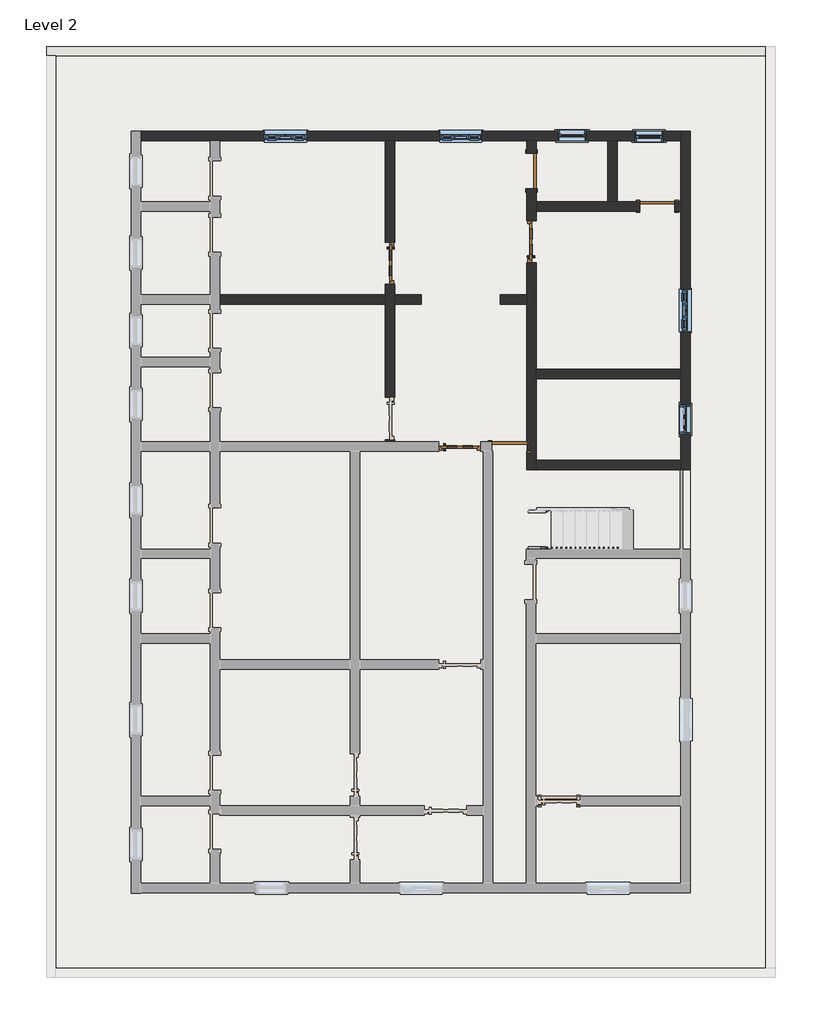
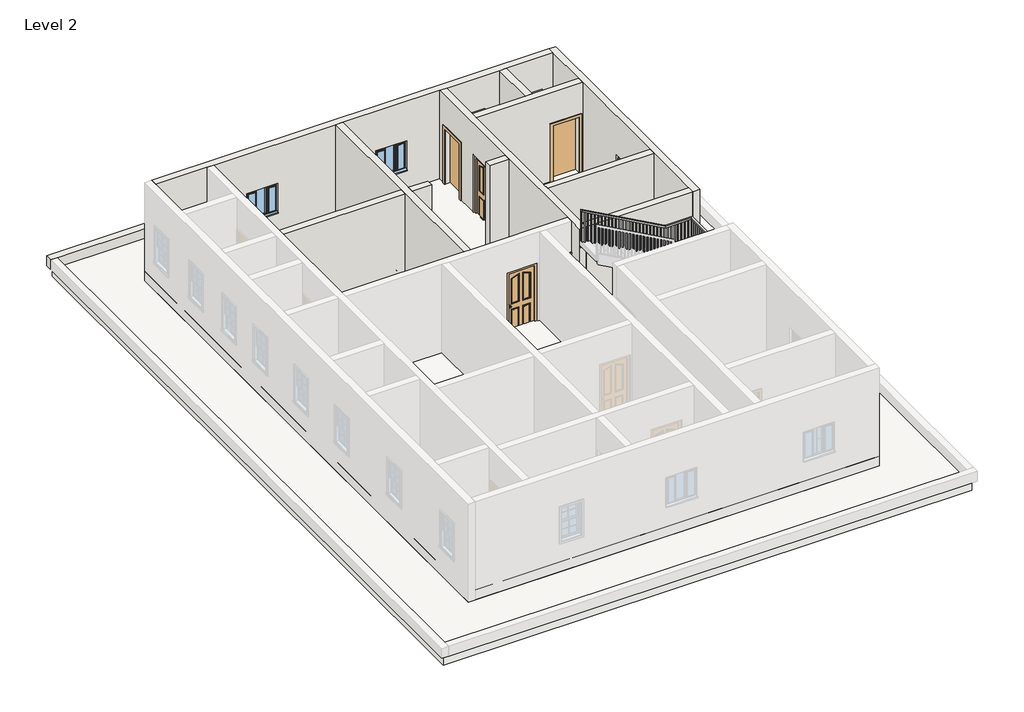
# One storey, part 2 of 3: 11 walls, 6 doors, 6 windows, 2 slabs, 1 railing, 1 roof.
"""IFC4 building model written with IfcOpenShell, lengths in millimetres."""

from ifc_helpers import new_model, si_unit, frame, origin, place, context, project, spatial, polyline, outline, extrude, faceted_brep, transform, mapped, element, save
from components import doors_extsgl_12_910x2110mm_9a09825e, doors_extsgl_12_910x2110mm_ece77ece, door_fadea3f2, window_679d2811, windows_tpl_w_glazing_cross_bars_910x910mm_4aa0f884

model = new_model("IFC4")

# Units and contexts
model_context = context("Model", 3, world=origin())
ifc_project = project(units=[si_unit("LENGTHUNIT", "METRE", prefix="MILLI")], contexts=[model_context])

# Site, building, storey
site = spatial("IfcSite", under=ifc_project)
building = spatial("IfcBuilding", under=site)
storey = spatial("IfcBuildingStorey", under=building, Name="Level 2", Elevation=3048.0)

# Doors
placement = place(None, origin())
doors_extsgl_12_910x2110mm_shape = doors_extsgl_12_910x2110mm_9a09825e(model_context)
element("IfcDoor", 1, ObjectType="Doors_ExtSgl_12 : 910x2110mm", at=placement, inside=storey, context=model_context, shape_type="MappedRepresentation", body=[
    mapped(doors_extsgl_12_910x2110mm_shape, transform((-4887.6876145, 4566.1404944, 3048.0), x_axis=(0.0, -1.0, 0.0), y_axis=(1.0, 0.0, 0.0), z_axis=(0.0, 0.0, 1.0))),
])
element("IfcDoor", 2, ObjectType="Doors_ExtSgl_12 : 910x2110mm", at=placement, inside=storey, context=model_context, shape_type="MappedRepresentation", body=[
    mapped(doors_extsgl_12_910x2110mm_shape, transform((-1839.6876145, 5029.6904944, 3048.0), x_axis=(0.0, 1.0, 0.0), y_axis=(-1.0, 0.0, 0.0), z_axis=(0.0, 0.0, 1.0))),
])
doors_extsgl_12_910x2110mm_2_shape = doors_extsgl_12_910x2110mm_ece77ece(model_context)
element("IfcDoor", 3, ObjectType="Doors_ExtSgl_12 : 910x2110mm", at=placement, inside=storey, context=model_context, shape_type="MappedRepresentation", body=[
    mapped(doors_extsgl_12_910x2110mm_2_shape, transform((-3389.0876145, 603.7404944, 3048.0), x_axis=(1.0, 0.0, 0.0), y_axis=(0.0, 1.0, 0.0), z_axis=(0.0, 0.0, 1.0))),
])
door_shape = door_fadea3f2(model_context)
element("IfcDoor", 4, ObjectType="Single-Flush : 30\" x 80\"", at=placement, inside=storey, context=model_context, shape_type="MappedRepresentation", body=[
    mapped(door_shape, transform((-1839.6876145, 6550.5154944, 3048.0), x_axis=(0.0, -1.0, 0.0), y_axis=(1.0, 0.0, 0.0), z_axis=(0.0, 0.0, 1.0))),
])
element("IfcDoor", 5, ObjectType="Single-Flush : 30\" x 80\"", at=placement, inside=storey, context=model_context, shape_type="MappedRepresentation", body=[
    mapped(door_shape, transform((878.1123855, 5791.6904944, 3048.0), x_axis=(1.0, 0.0, 0.0), y_axis=(0.0, 1.0, 0.0), z_axis=(0.0, 0.0, 1.0))),
])
element("IfcDoor", 6, ObjectType="Single-Flush : 30\" x 80\"", at=placement, inside=storey, context=model_context, shape_type="MappedRepresentation", body=[
    mapped(door_shape, transform((-2309.5876145, 603.7404944, 3048.0), x_axis=(1.0, 0.0, 0.0), y_axis=(0.0, 1.0, 0.0), z_axis=(0.0, 0.0, 1.0))),
])

# Railing
element("IfcRailing", 7, ObjectType="Handrail - Rectangular", at=placement, inside=storey, context=model_context, shape_type="SolidModel", body=[
    faceted_brep([(-1903.1876145, -1555.2595056, 4099.56), (-1903.1876145, -1555.2595056, 4041.4879132), (-1903.1876145, -1606.0595056, 4041.4879132), (-1903.1876145, -1606.0595056, 4099.56), (325.4830625, -1555.2595056, 5334.0), (338.6121628, -1555.2595056, 5283.2), (338.6121628, -1606.0595056, 5283.2), (325.4830625, -1606.0595056, 5334.0), (1322.6123855, -1555.2595056, 5334.0), (1322.6123855, -1555.2595056, 5283.2), (1373.4123855, -1606.0595056, 5283.2), (1373.4123855, -1606.0595056, 5334.0), (1322.6123855, 57.6404944, 5334.0), (1322.6123855, 57.6404944, 5283.2), (1373.4123855, 108.4404944, 5283.2), (1373.4123855, 108.4404944, 5334.0), (573.1131377, 57.6404944, 5334.0), (559.9840375, 57.6404944, 5283.2), (559.9840375, 108.4404944, 5283.2), (573.1131377, 108.4404944, 5334.0), (-1903.1876145, 57.6404944, 6705.6), (-1903.1876145, 108.4404944, 6705.6), (-1903.1876145, 108.4404944, 6647.5279132), (-1903.1876145, 57.6404944, 6647.5279132)], [[[0, 1, 2, 3]], [[1, 0, 4, 5]], [[2, 1, 5, 6]], [[3, 2, 6, 7]], [[0, 3, 7, 4]], [[5, 4, 8, 9]], [[6, 5, 9, 10]], [[7, 6, 10, 11]], [[4, 7, 11, 8]], [[9, 8, 12, 13]], [[10, 9, 13, 14]], [[11, 10, 14, 15]], [[8, 11, 15, 12]], [[13, 12, 16, 17]], [[14, 13, 17, 18]], [[15, 14, 18, 19]], [[12, 15, 19, 16]], [[20, 21, 22, 23]], [[17, 16, 20, 23]], [[18, 17, 23, 22]], [[19, 18, 22, 21]], [[16, 19, 21, 20]]]),
    extrude(outline(polyline([(6585.9768073, -1792.0626145), (6596.5284254, -1811.1126145), (5654.04, -1811.1126145), (5654.04, -1792.0626145), (6585.9768073, -1792.0626145)])), frame((0.0, 73.5154944, 0.0), z_axis=(0.0, 1.0, 0.0), x_axis=(0.0, 0.0, 1.0)), (0.0, 0.0, 1.0), 19.05),
    extrude(outline(polyline([(6529.7015104, -1690.4626145), (6540.2531286, -1709.5126145), (5654.04, -1709.5126145), (5654.04, -1690.4626145), (6529.7015104, -1690.4626145)])), frame((0.0, 73.5154944, 0.0), z_axis=(0.0, 1.0, 0.0), x_axis=(0.0, 0.0, 1.0)), (0.0, 0.0, 1.0), 19.05),
    extrude(outline(polyline([(6473.4262135, -1588.8626145), (6483.9778317, -1607.9126145), (5516.88, -1607.9126145), (5516.88, -1588.8626145), (6473.4262135, -1588.8626145)])), frame((0.0, 73.5154944, 0.0), z_axis=(0.0, 1.0, 0.0), x_axis=(0.0, 0.0, 1.0)), (0.0, 0.0, 1.0), 19.05),
    extrude(outline(polyline([(6417.1509166, -1487.2626145), (6427.7025348, -1506.3126145), (5516.88, -1506.3126145), (5516.88, -1487.2626145), (6417.1509166, -1487.2626145)])), frame((0.0, 73.5154944, 0.0), z_axis=(0.0, 1.0, 0.0), x_axis=(0.0, 0.0, 1.0)), (0.0, 0.0, 1.0), 19.05),
    extrude(outline(polyline([(6360.8756198, -1385.6626145), (6371.4272379, -1404.7126145), (5379.72, -1404.7126145), (5379.72, -1385.6626145), (6360.8756198, -1385.6626145)])), frame((0.0, 73.5154944, 0.0), z_axis=(0.0, 1.0, 0.0), x_axis=(0.0, 0.0, 1.0)), (0.0, 0.0, 1.0), 19.05),
    extrude(outline(polyline([(6304.6003229, -1284.0626145), (6315.151941, -1303.1126145), (5379.72, -1303.1126145), (5379.72, -1284.0626145), (6304.6003229, -1284.0626145)])), frame((0.0, 73.5154944, 0.0), z_axis=(0.0, 1.0, 0.0), x_axis=(0.0, 0.0, 1.0)), (0.0, 0.0, 1.0), 19.05),
    extrude(outline(polyline([(6248.325026, -1182.4626145), (6258.8766442, -1201.5126145), (5379.72, -1201.5126145), (5379.72, -1182.4626145), (6248.325026, -1182.4626145)])), frame((0.0, 73.5154944, 0.0), z_axis=(0.0, 1.0, 0.0), x_axis=(0.0, 0.0, 1.0)), (0.0, 0.0, 1.0), 19.05),
    extrude(outline(polyline([(6192.0497291, -1080.8626145), (6202.6013473, -1099.9126145), (5242.56, -1099.9126145), (5242.56, -1080.8626145), (6192.0497291, -1080.8626145)])), frame((0.0, 73.5154944, 0.0), z_axis=(0.0, 1.0, 0.0), x_axis=(0.0, 0.0, 1.0)), (0.0, 0.0, 1.0), 19.05),
    extrude(outline(polyline([(6135.7744322, -979.2626145), (6146.3260504, -998.3126145), (5242.56, -998.3126145), (5242.56, -979.2626145), (6135.7744322, -979.2626145)])), frame((0.0, 73.5154944, 0.0), z_axis=(0.0, 1.0, 0.0), x_axis=(0.0, 0.0, 1.0)), (0.0, 0.0, 1.0), 19.05),
    extrude(outline(polyline([(6079.4991354, -877.6626145), (6090.0507535, -896.7126145), (5105.4, -896.7126145), (5105.4, -877.6626145), (6079.4991354, -877.6626145)])), frame((0.0, 73.5154944, 0.0), z_axis=(0.0, 1.0, 0.0), x_axis=(0.0, 0.0, 1.0)), (0.0, 0.0, 1.0), 19.05),
    extrude(outline(polyline([(6023.2238385, -776.0626145), (6033.7754566, -795.1126145), (5105.4, -795.1126145), (5105.4, -776.0626145), (6023.2238385, -776.0626145)])), frame((0.0, 73.5154944, 0.0), z_axis=(0.0, 1.0, 0.0), x_axis=(0.0, 0.0, 1.0)), (0.0, 0.0, 1.0), 19.05),
    extrude(outline(polyline([(5966.9485416, -674.4626145), (5977.5001598, -693.5126145), (5105.4, -693.5126145), (5105.4, -674.4626145), (5966.9485416, -674.4626145)])), frame((0.0, 73.5154944, 0.0), z_axis=(0.0, 1.0, 0.0), x_axis=(0.0, 0.0, 1.0)), (0.0, 0.0, 1.0), 19.05),
    extrude(outline(polyline([(5910.6732447, -572.8626145), (5921.2248629, -591.9126145), (4968.24, -591.9126145), (4968.24, -572.8626145), (5910.6732447, -572.8626145)])), frame((0.0, 73.5154944, 0.0), z_axis=(0.0, 1.0, 0.0), x_axis=(0.0, 0.0, 1.0)), (0.0, 0.0, 1.0), 19.05),
    extrude(outline(polyline([(5854.3979478, -471.2626145), (5864.949566, -490.3126145), (4968.24, -490.3126145), (4968.24, -471.2626145), (5854.3979478, -471.2626145)])), frame((0.0, 73.5154944, 0.0), z_axis=(0.0, 1.0, 0.0), x_axis=(0.0, 0.0, 1.0)), (0.0, 0.0, 1.0), 19.05),
    extrude(outline(polyline([(5798.1226509, -369.6626145), (5808.6742691, -388.7126145), (4831.08, -388.7126145), (4831.08, -369.6626145), (5798.1226509, -369.6626145)])), frame((0.0, 73.5154944, 0.0), z_axis=(0.0, 1.0, 0.0), x_axis=(0.0, 0.0, 1.0)), (0.0, 0.0, 1.0), 19.05),
    extrude(outline(polyline([(5741.8473541, -268.0626145), (5752.3989722, -287.1126145), (4831.08, -287.1126145), (4831.08, -268.0626145), (5741.8473541, -268.0626145)])), frame((0.0, 73.5154944, 0.0), z_axis=(0.0, 1.0, 0.0), x_axis=(0.0, 0.0, 1.0)), (0.0, 0.0, 1.0), 19.05),
    extrude(outline(polyline([(5685.5720572, -166.4626145), (5696.1236754, -185.5126145), (4831.08, -185.5126145), (4831.08, -166.4626145), (5685.5720572, -166.4626145)])), frame((0.0, 73.5154944, 0.0), z_axis=(0.0, 1.0, 0.0), x_axis=(0.0, 0.0, 1.0)), (0.0, 0.0, 1.0), 19.05),
    extrude(outline(polyline([(5629.2967603, -64.8626145), (5639.8483785, -83.9126145), (4693.92, -83.9126145), (4693.92, -64.8626145), (5629.2967603, -64.8626145)])), frame((0.0, 73.5154944, 0.0), z_axis=(0.0, 1.0, 0.0), x_axis=(0.0, 0.0, 1.0)), (0.0, 0.0, 1.0), 19.05),
    extrude(outline(polyline([(5573.0214634, 36.7373855), (5583.5730816, 17.6873855), (4693.92, 17.6873855), (4693.92, 36.7373855), (5573.0214634, 36.7373855)])), frame((0.0, 73.5154944, 0.0), z_axis=(0.0, 1.0, 0.0), x_axis=(0.0, 0.0, 1.0)), (0.0, 0.0, 1.0), 19.05),
    extrude(outline(polyline([(5516.7461665, 138.3373855), (5527.2977847, 119.2873855), (4556.76, 119.2873855), (4556.76, 138.3373855), (5516.7461665, 138.3373855)])), frame((0.0, 73.5154944, 0.0), z_axis=(0.0, 1.0, 0.0), x_axis=(0.0, 0.0, 1.0)), (0.0, 0.0, 1.0), 19.05),
    extrude(outline(polyline([(5460.4708697, 239.9373855), (5471.0224878, 220.8873855), (4556.76, 220.8873855), (4556.76, 239.9373855), (5460.4708697, 239.9373855)])), frame((0.0, 73.5154944, 0.0), z_axis=(0.0, 1.0, 0.0), x_axis=(0.0, 0.0, 1.0)), (0.0, 0.0, 1.0), 19.05),
    extrude(outline(polyline([(5404.1955728, 341.5373855), (5414.7471909, 322.4873855), (4419.6, 322.4873855), (4419.6, 341.5373855), (5404.1955728, 341.5373855)])), frame((0.0, 73.5154944, 0.0), z_axis=(0.0, 1.0, 0.0), x_axis=(0.0, 0.0, 1.0)), (0.0, 0.0, 1.0), 19.05),
    extrude(outline(polyline([(5347.9202759, 443.1373855), (5358.4718941, 424.0873855), (4419.6, 424.0873855), (4419.6, 443.1373855), (5347.9202759, 443.1373855)])), frame((0.0, 73.5154944, 0.0), z_axis=(0.0, 1.0, 0.0), x_axis=(0.0, 0.0, 1.0)), (0.0, 0.0, 1.0), 19.05),
    extrude(outline(polyline([(5291.644979, 544.7373855), (5302.1965972, 525.6873855), (4419.6, 525.6873855), (4419.6, 544.7373855), (5291.644979, 544.7373855)])), frame((0.0, 73.5154944, 0.0), z_axis=(0.0, 1.0, 0.0), x_axis=(0.0, 0.0, 1.0)), (0.0, 0.0, 1.0), 19.05),
    extrude(outline(polyline([(646.3373855, 92.5654944), (646.3373855, 73.5154944), (627.2873855, 73.5154944), (627.2873855, 92.5654944), (646.3373855, 92.5654944)])), frame((0.0, 0.0, 4419.6), z_axis=(0.0, 0.0, 1.0), x_axis=(1.0, 0.0, 0.0)), (0.0, 0.0, 1.0), 863.6),
    extrude(outline(polyline([(747.9373855, 92.5654944), (747.9373855, 73.5154944), (728.8873855, 73.5154944), (728.8873855, 92.5654944), (747.9373855, 92.5654944)])), frame((0.0, 0.0, 4419.6), z_axis=(0.0, 0.0, 1.0), x_axis=(1.0, 0.0, 0.0)), (0.0, 0.0, 1.0), 863.6),
    extrude(outline(polyline([(849.5373855, 92.5654944), (849.5373855, 73.5154944), (830.4873855, 73.5154944), (830.4873855, 92.5654944), (849.5373855, 92.5654944)])), frame((0.0, 0.0, 4419.6), z_axis=(0.0, 0.0, 1.0), x_axis=(1.0, 0.0, 0.0)), (0.0, 0.0, 1.0), 863.6),
    extrude(outline(polyline([(951.1373855, 92.5654944), (951.1373855, 73.5154944), (932.0873855, 73.5154944), (932.0873855, 92.5654944), (951.1373855, 92.5654944)])), frame((0.0, 0.0, 4419.6), z_axis=(0.0, 0.0, 1.0), x_axis=(1.0, 0.0, 0.0)), (0.0, 0.0, 1.0), 863.6),
    extrude(outline(polyline([(1052.7373855, 92.5654944), (1052.7373855, 73.5154944), (1033.6873855, 73.5154944), (1033.6873855, 92.5654944), (1052.7373855, 92.5654944)])), frame((0.0, 0.0, 4419.6), z_axis=(0.0, 0.0, 1.0), x_axis=(1.0, 0.0, 0.0)), (0.0, 0.0, 1.0), 863.6),
    extrude(outline(polyline([(1154.3373855, 92.5654944), (1154.3373855, 73.5154944), (1135.2873855, 73.5154944), (1135.2873855, 92.5654944), (1154.3373855, 92.5654944)])), frame((0.0, 0.0, 4419.6), z_axis=(0.0, 0.0, 1.0), x_axis=(1.0, 0.0, 0.0)), (0.0, 0.0, 1.0), 863.6),
    extrude(outline(polyline([(1255.9373855, 92.5654944), (1255.9373855, 73.5154944), (1236.8873855, 73.5154944), (1236.8873855, 92.5654944), (1255.9373855, 92.5654944)])), frame((0.0, 0.0, 4419.6), z_axis=(0.0, 0.0, 1.0), x_axis=(1.0, 0.0, 0.0)), (0.0, 0.0, 1.0), 863.6),
    extrude(outline(polyline([(1357.5373855, 35.4154944), (1338.4873855, 35.4154944), (1338.4873855, 54.4654944), (1357.5373855, 54.4654944), (1357.5373855, 35.4154944)])), frame((0.0, 0.0, 4419.6), z_axis=(0.0, 0.0, 1.0), x_axis=(1.0, 0.0, 0.0)), (0.0, 0.0, 1.0), 863.6),
    extrude(outline(polyline([(1357.5373855, -66.1845056), (1338.4873855, -66.1845056), (1338.4873855, -47.1345056), (1357.5373855, -47.1345056), (1357.5373855, -66.1845056)])), frame((0.0, 0.0, 4419.6), z_axis=(0.0, 0.0, 1.0), x_axis=(1.0, 0.0, 0.0)), (0.0, 0.0, 1.0), 863.6),
    extrude(outline(polyline([(1357.5373855, -167.7845056), (1338.4873855, -167.7845056), (1338.4873855, -148.7345056), (1357.5373855, -148.7345056), (1357.5373855, -167.7845056)])), frame((0.0, 0.0, 4419.6), z_axis=(0.0, 0.0, 1.0), x_axis=(1.0, 0.0, 0.0)), (0.0, 0.0, 1.0), 863.6),
    extrude(outline(polyline([(1357.5373855, -269.3845056), (1338.4873855, -269.3845056), (1338.4873855, -250.3345056), (1357.5373855, -250.3345056), (1357.5373855, -269.3845056)])), frame((0.0, 0.0, 4419.6), z_axis=(0.0, 0.0, 1.0), x_axis=(1.0, 0.0, 0.0)), (0.0, 0.0, 1.0), 863.6),
    extrude(outline(polyline([(1357.5373855, -370.9845056), (1338.4873855, -370.9845056), (1338.4873855, -351.9345056), (1357.5373855, -351.9345056), (1357.5373855, -370.9845056)])), frame((0.0, 0.0, 4419.6), z_axis=(0.0, 0.0, 1.0), x_axis=(1.0, 0.0, 0.0)), (0.0, 0.0, 1.0), 863.6),
    extrude(outline(polyline([(1357.5373855, -472.5845056), (1338.4873855, -472.5845056), (1338.4873855, -453.5345056), (1357.5373855, -453.5345056), (1357.5373855, -472.5845056)])), frame((0.0, 0.0, 4419.6), z_axis=(0.0, 0.0, 1.0), x_axis=(1.0, 0.0, 0.0)), (0.0, 0.0, 1.0), 863.6),
    extrude(outline(polyline([(1357.5373855, -574.1845056), (1338.4873855, -574.1845056), (1338.4873855, -555.1345056), (1357.5373855, -555.1345056), (1357.5373855, -574.1845056)])), frame((0.0, 0.0, 4419.6), z_axis=(0.0, 0.0, 1.0), x_axis=(1.0, 0.0, 0.0)), (0.0, 0.0, 1.0), 863.6),
    extrude(outline(polyline([(1357.5373855, -675.7845056), (1338.4873855, -675.7845056), (1338.4873855, -656.7345056), (1357.5373855, -656.7345056), (1357.5373855, -675.7845056)])), frame((0.0, 0.0, 4419.6), z_axis=(0.0, 0.0, 1.0), x_axis=(1.0, 0.0, 0.0)), (0.0, 0.0, 1.0), 863.6),
    extrude(outline(polyline([(1357.5373855, -777.3845056), (1338.4873855, -777.3845056), (1338.4873855, -758.3345056), (1357.5373855, -758.3345056), (1357.5373855, -777.3845056)])), frame((0.0, 0.0, 4419.6), z_axis=(0.0, 0.0, 1.0), x_axis=(1.0, 0.0, 0.0)), (0.0, 0.0, 1.0), 863.6),
    extrude(outline(polyline([(1357.5373855, -878.9845056), (1338.4873855, -878.9845056), (1338.4873855, -859.9345056), (1357.5373855, -859.9345056), (1357.5373855, -878.9845056)])), frame((0.0, 0.0, 4419.6), z_axis=(0.0, 0.0, 1.0), x_axis=(1.0, 0.0, 0.0)), (0.0, 0.0, 1.0), 863.6),
    extrude(outline(polyline([(1357.5373855, -980.5845056), (1338.4873855, -980.5845056), (1338.4873855, -961.5345056), (1357.5373855, -961.5345056), (1357.5373855, -980.5845056)])), frame((0.0, 0.0, 4419.6), z_axis=(0.0, 0.0, 1.0), x_axis=(1.0, 0.0, 0.0)), (0.0, 0.0, 1.0), 863.6),
    extrude(outline(polyline([(1357.5373855, -1082.1845056), (1338.4873855, -1082.1845056), (1338.4873855, -1063.1345056), (1357.5373855, -1063.1345056), (1357.5373855, -1082.1845056)])), frame((0.0, 0.0, 4419.6), z_axis=(0.0, 0.0, 1.0), x_axis=(1.0, 0.0, 0.0)), (0.0, 0.0, 1.0), 863.6),
    extrude(outline(polyline([(1357.5373855, -1183.7845056), (1338.4873855, -1183.7845056), (1338.4873855, -1164.7345056), (1357.5373855, -1164.7345056), (1357.5373855, -1183.7845056)])), frame((0.0, 0.0, 4419.6), z_axis=(0.0, 0.0, 1.0), x_axis=(1.0, 0.0, 0.0)), (0.0, 0.0, 1.0), 863.6),
    extrude(outline(polyline([(1357.5373855, -1285.3845056), (1338.4873855, -1285.3845056), (1338.4873855, -1266.3345056), (1357.5373855, -1266.3345056), (1357.5373855, -1285.3845056)])), frame((0.0, 0.0, 4419.6), z_axis=(0.0, 0.0, 1.0), x_axis=(1.0, 0.0, 0.0)), (0.0, 0.0, 1.0), 863.6),
    extrude(outline(polyline([(1357.5373855, -1386.9845056), (1338.4873855, -1386.9845056), (1338.4873855, -1367.9345056), (1357.5373855, -1367.9345056), (1357.5373855, -1386.9845056)])), frame((0.0, 0.0, 4419.6), z_axis=(0.0, 0.0, 1.0), x_axis=(1.0, 0.0, 0.0)), (0.0, 0.0, 1.0), 863.6),
    extrude(outline(polyline([(1357.5373855, -1488.5845056), (1338.4873855, -1488.5845056), (1338.4873855, -1469.5345056), (1357.5373855, -1469.5345056), (1357.5373855, -1488.5845056)])), frame((0.0, 0.0, 4419.6), z_axis=(0.0, 0.0, 1.0), x_axis=(1.0, 0.0, 0.0)), (0.0, 0.0, 1.0), 863.6),
    extrude(outline(polyline([(1236.8873855, -1590.1845056), (1236.8873855, -1571.1345056), (1255.9373855, -1571.1345056), (1255.9373855, -1590.1845056), (1236.8873855, -1590.1845056)])), frame((0.0, 0.0, 4419.6), z_axis=(0.0, 0.0, 1.0), x_axis=(1.0, 0.0, 0.0)), (0.0, 0.0, 1.0), 863.6),
    extrude(outline(polyline([(1135.2873855, -1590.1845056), (1135.2873855, -1571.1345056), (1154.3373855, -1571.1345056), (1154.3373855, -1590.1845056), (1135.2873855, -1590.1845056)])), frame((0.0, 0.0, 4419.6), z_axis=(0.0, 0.0, 1.0), x_axis=(1.0, 0.0, 0.0)), (0.0, 0.0, 1.0), 863.6),
    extrude(outline(polyline([(1033.6873855, -1590.1845056), (1033.6873855, -1571.1345056), (1052.7373855, -1571.1345056), (1052.7373855, -1590.1845056), (1033.6873855, -1590.1845056)])), frame((0.0, 0.0, 4419.6), z_axis=(0.0, 0.0, 1.0), x_axis=(1.0, 0.0, 0.0)), (0.0, 0.0, 1.0), 863.6),
    extrude(outline(polyline([(932.0873855, -1590.1845056), (932.0873855, -1571.1345056), (951.1373855, -1571.1345056), (951.1373855, -1590.1845056), (932.0873855, -1590.1845056)])), frame((0.0, 0.0, 4419.6), z_axis=(0.0, 0.0, 1.0), x_axis=(1.0, 0.0, 0.0)), (0.0, 0.0, 1.0), 863.6),
    extrude(outline(polyline([(830.4873855, -1590.1845056), (830.4873855, -1571.1345056), (849.5373855, -1571.1345056), (849.5373855, -1590.1845056), (830.4873855, -1590.1845056)])), frame((0.0, 0.0, 4419.6), z_axis=(0.0, 0.0, 1.0), x_axis=(1.0, 0.0, 0.0)), (0.0, 0.0, 1.0), 863.6),
    extrude(outline(polyline([(728.8873855, -1590.1845056), (728.8873855, -1571.1345056), (747.9373855, -1571.1345056), (747.9373855, -1590.1845056), (728.8873855, -1590.1845056)])), frame((0.0, 0.0, 4419.6), z_axis=(0.0, 0.0, 1.0), x_axis=(1.0, 0.0, 0.0)), (0.0, 0.0, 1.0), 863.6),
    extrude(outline(polyline([(627.2873855, -1590.1845056), (627.2873855, -1571.1345056), (646.3373855, -1571.1345056), (646.3373855, -1590.1845056), (627.2873855, -1590.1845056)])), frame((0.0, 0.0, 4419.6), z_axis=(0.0, 0.0, 1.0), x_axis=(1.0, 0.0, 0.0)), (0.0, 0.0, 1.0), 863.6),
    extrude(outline(polyline([(525.6873855, -1590.1845056), (525.6873855, -1571.1345056), (544.7373855, -1571.1345056), (544.7373855, -1590.1845056), (525.6873855, -1590.1845056)])), frame((0.0, 0.0, 4419.6), z_axis=(0.0, 0.0, 1.0), x_axis=(1.0, 0.0, 0.0)), (0.0, 0.0, 1.0), 863.6),
    extrude(outline(polyline([(424.0873855, -1590.1845056), (424.0873855, -1571.1345056), (443.1373855, -1571.1345056), (443.1373855, -1590.1845056), (424.0873855, -1590.1845056)])), frame((0.0, 0.0, 4419.6), z_axis=(0.0, 0.0, 1.0), x_axis=(1.0, 0.0, 0.0)), (0.0, 0.0, 1.0), 863.6),
    extrude(outline(polyline([(322.4873855, -1590.1845056), (322.4873855, -1571.1345056), (341.5373855, -1571.1345056), (341.5373855, -1590.1845056), (322.4873855, -1590.1845056)])), frame((0.0, 0.0, 4419.6), z_axis=(0.0, 0.0, 1.0), x_axis=(1.0, 0.0, 0.0)), (0.0, 0.0, 1.0), 863.6),
    extrude(outline(polyline([(5228.5449568, 239.9373855), (5217.9933387, 220.8873855), (4282.44, 220.8873855), (4282.44, 239.9373855), (5228.5449568, 239.9373855)])), frame((0.0, -1590.1845056, 0.0), z_axis=(0.0, 1.0, 0.0), x_axis=(0.0, 0.0, 1.0)), (0.0, 0.0, 1.0), 19.05),
    extrude(outline(polyline([(5172.2696599, 138.3373855), (5161.7180418, 119.2873855), (4282.44, 119.2873855), (4282.44, 138.3373855), (5172.2696599, 138.3373855)])), frame((0.0, -1590.1845056, 0.0), z_axis=(0.0, 1.0, 0.0), x_axis=(0.0, 0.0, 1.0)), (0.0, 0.0, 1.0), 19.05),
    extrude(outline(polyline([(5115.9943631, 36.7373855), (5105.4427449, 17.6873855), (4145.28, 17.6873855), (4145.28, 36.7373855), (5115.9943631, 36.7373855)])), frame((0.0, -1590.1845056, 0.0), z_axis=(0.0, 1.0, 0.0), x_axis=(0.0, 0.0, 1.0)), (0.0, 0.0, 1.0), 19.05),
    extrude(outline(polyline([(5059.7190662, -64.8626145), (5049.167448, -83.9126145), (4145.28, -83.9126145), (4145.28, -64.8626145), (5059.7190662, -64.8626145)])), frame((0.0, -1590.1845056, 0.0), z_axis=(0.0, 1.0, 0.0), x_axis=(0.0, 0.0, 1.0)), (0.0, 0.0, 1.0), 19.05),
    extrude(outline(polyline([(5003.4437693, -166.4626145), (4992.8921511, -185.5126145), (4008.12, -185.5126145), (4008.12, -166.4626145), (5003.4437693, -166.4626145)])), frame((0.0, -1590.1845056, 0.0), z_axis=(0.0, 1.0, 0.0), x_axis=(0.0, 0.0, 1.0)), (0.0, 0.0, 1.0), 19.05),
    extrude(outline(polyline([(4947.1684724, -268.0626145), (4936.6168543, -287.1126145), (4008.12, -287.1126145), (4008.12, -268.0626145), (4947.1684724, -268.0626145)])), frame((0.0, -1590.1845056, 0.0), z_axis=(0.0, 1.0, 0.0), x_axis=(0.0, 0.0, 1.0)), (0.0, 0.0, 1.0), 19.05),
    extrude(outline(polyline([(4890.8931755, -369.6626145), (4880.3415574, -388.7126145), (4008.12, -388.7126145), (4008.12, -369.6626145), (4890.8931755, -369.6626145)])), frame((0.0, -1590.1845056, 0.0), z_axis=(0.0, 1.0, 0.0), x_axis=(0.0, 0.0, 1.0)), (0.0, 0.0, 1.0), 19.05),
    extrude(outline(polyline([(4834.6178787, -471.2626145), (4824.0662605, -490.3126145), (3870.96, -490.3126145), (3870.96, -471.2626145), (4834.6178787, -471.2626145)])), frame((0.0, -1590.1845056, 0.0), z_axis=(0.0, 1.0, 0.0), x_axis=(0.0, 0.0, 1.0)), (0.0, 0.0, 1.0), 19.05),
    extrude(outline(polyline([(4778.3425818, -572.8626145), (4767.7909636, -591.9126145), (3870.96, -591.9126145), (3870.96, -572.8626145), (4778.3425818, -572.8626145)])), frame((0.0, -1590.1845056, 0.0), z_axis=(0.0, 1.0, 0.0), x_axis=(0.0, 0.0, 1.0)), (0.0, 0.0, 1.0), 19.05),
    extrude(outline(polyline([(4722.0672849, -674.4626145), (4711.5156667, -693.5126145), (3733.8, -693.5126145), (3733.8, -674.4626145), (4722.0672849, -674.4626145)])), frame((0.0, -1590.1845056, 0.0), z_axis=(0.0, 1.0, 0.0), x_axis=(0.0, 0.0, 1.0)), (0.0, 0.0, 1.0), 19.05),
    extrude(outline(polyline([(4665.791988, -776.0626145), (4655.2403699, -795.1126145), (3733.8, -795.1126145), (3733.8, -776.0626145), (4665.791988, -776.0626145)])), frame((0.0, -1590.1845056, 0.0), z_axis=(0.0, 1.0, 0.0), x_axis=(0.0, 0.0, 1.0)), (0.0, 0.0, 1.0), 19.05),
    extrude(outline(polyline([(4609.5166911, -877.6626145), (4598.965073, -896.7126145), (3733.8, -896.7126145), (3733.8, -877.6626145), (4609.5166911, -877.6626145)])), frame((0.0, -1590.1845056, 0.0), z_axis=(0.0, 1.0, 0.0), x_axis=(0.0, 0.0, 1.0)), (0.0, 0.0, 1.0), 19.05),
    extrude(outline(polyline([(4553.2413943, -979.2626145), (4542.6897761, -998.3126145), (3596.64, -998.3126145), (3596.64, -979.2626145), (4553.2413943, -979.2626145)])), frame((0.0, -1590.1845056, 0.0), z_axis=(0.0, 1.0, 0.0), x_axis=(0.0, 0.0, 1.0)), (0.0, 0.0, 1.0), 19.05),
    extrude(outline(polyline([(4496.9660974, -1080.8626145), (4486.4144792, -1099.9126145), (3596.64, -1099.9126145), (3596.64, -1080.8626145), (4496.9660974, -1080.8626145)])), frame((0.0, -1590.1845056, 0.0), z_axis=(0.0, 1.0, 0.0), x_axis=(0.0, 0.0, 1.0)), (0.0, 0.0, 1.0), 19.05),
    extrude(outline(polyline([(4440.6908005, -1182.4626145), (4430.1391823, -1201.5126145), (3459.48, -1201.5126145), (3459.48, -1182.4626145), (4440.6908005, -1182.4626145)])), frame((0.0, -1590.1845056, 0.0), z_axis=(0.0, 1.0, 0.0), x_axis=(0.0, 0.0, 1.0)), (0.0, 0.0, 1.0), 19.05),
    extrude(outline(polyline([(4384.4155036, -1284.0626145), (4373.8638855, -1303.1126145), (3459.48, -1303.1126145), (3459.48, -1284.0626145), (4384.4155036, -1284.0626145)])), frame((0.0, -1590.1845056, 0.0), z_axis=(0.0, 1.0, 0.0), x_axis=(0.0, 0.0, 1.0)), (0.0, 0.0, 1.0), 19.05),
    extrude(outline(polyline([(4328.1402067, -1385.6626145), (4317.5885886, -1404.7126145), (3459.48, -1404.7126145), (3459.48, -1385.6626145), (4328.1402067, -1385.6626145)])), frame((0.0, -1590.1845056, 0.0), z_axis=(0.0, 1.0, 0.0), x_axis=(0.0, 0.0, 1.0)), (0.0, 0.0, 1.0), 19.05),
    extrude(outline(polyline([(4271.8649099, -1487.2626145), (4261.3132917, -1506.3126145), (3322.32, -1506.3126145), (3322.32, -1487.2626145), (4271.8649099, -1487.2626145)])), frame((0.0, -1590.1845056, 0.0), z_axis=(0.0, 1.0, 0.0), x_axis=(0.0, 0.0, 1.0)), (0.0, 0.0, 1.0), 19.05),
    extrude(outline(polyline([(4215.589613, -1588.8626145), (4205.0379948, -1607.9126145), (3322.32, -1607.9126145), (3322.32, -1588.8626145), (4215.589613, -1588.8626145)])), frame((0.0, -1590.1845056, 0.0), z_axis=(0.0, 1.0, 0.0), x_axis=(0.0, 0.0, 1.0)), (0.0, 0.0, 1.0), 19.05),
    extrude(outline(polyline([(4159.3143161, -1690.4626145), (4148.7626979, -1709.5126145), (3185.16, -1709.5126145), (3185.16, -1690.4626145), (4159.3143161, -1690.4626145)])), frame((0.0, -1590.1845056, 0.0), z_axis=(0.0, 1.0, 0.0), x_axis=(0.0, 0.0, 1.0)), (0.0, 0.0, 1.0), 19.05),
    extrude(outline(polyline([(4103.0390192, -1792.0626145), (4092.487401, -1811.1126145), (3185.16, -1811.1126145), (3185.16, -1792.0626145), (4103.0390192, -1792.0626145)])), frame((0.0, -1590.1845056, 0.0), z_axis=(0.0, 1.0, 0.0), x_axis=(0.0, 0.0, 1.0)), (0.0, 0.0, 1.0), 19.05),
    extrude(outline(polyline([(1357.5373855, 73.5154944), (1338.4873855, 73.5154944), (1338.4873855, 92.5654944), (1357.5373855, 92.5654944), (1357.5373855, 73.5154944)])), frame((0.0, 0.0, 4419.6), z_axis=(0.0, 0.0, 1.0), x_axis=(1.0, 0.0, 0.0)), (0.0, 0.0, 1.0), 863.6),
    extrude(outline(polyline([(1338.4873855, -1590.1845056), (1338.4873855, -1571.1345056), (1357.5373855, -1571.1345056), (1357.5373855, -1590.1845056), (1338.4873855, -1590.1845056)])), frame((0.0, 0.0, 4419.6), z_axis=(0.0, 0.0, 1.0), x_axis=(1.0, 0.0, 0.0)), (0.0, 0.0, 1.0), 863.6),
    extrude(outline(polyline([(6636.9762951, -1884.1376145), (6647.5279132, -1903.1876145), (5654.04, -1903.1876145), (5654.04, -1884.1376145), (6636.9762951, -1884.1376145)])), frame((0.0, 73.5154944, 0.0), z_axis=(0.0, 1.0, 0.0), x_axis=(0.0, 0.0, 1.0)), (0.0, 0.0, 1.0), 19.05),
    extrude(outline(polyline([(4052.0395314, -1884.1376145), (4041.4879132, -1903.1876145), (3185.16, -1903.1876145), (3185.16, -1884.1376145), (4052.0395314, -1884.1376145)])), frame((0.0, -1590.1845056, 0.0), z_axis=(0.0, 1.0, 0.0), x_axis=(0.0, 0.0, 1.0)), (0.0, 0.0, 1.0), 19.05),
])

# Roof
element("IfcRoof", 8, ObjectType="Generic - 12\"", at=placement, inside=storey, context=model_context, shape_type="SweptSolid", body=[
    extrude(outline(polyline([(-10475.6876145, 7410.9404944), (1589.3123855, 7410.9404944), (1589.3123855, -9022.8595056), (-10475.6876145, -9022.8595056), (-10475.6876145, 7410.9404944)])), frame((0.0, 0.0, 3048.0), z_axis=(0.0, 0.0, 1.0), x_axis=(1.0, 0.0, 0.0)), (0.0, 0.0, 1.0), 304.8),
])

# Slabs
element("IfcSlab", 9, ObjectType="Generic - 12\"", at=placement, inside=storey, context=model_context, shape_type="SweptSolid", body=[
    extrude(outline(polyline([(1589.3123855, 7410.9404944), (1589.3123855, -9022.8595056), (-10475.6876145, -9022.8595056), (-10475.6876145, 7410.9404944), (1589.3123855, 7410.9404944)])), frame((0.0, 0.0, 2743.2), z_axis=(0.0, 0.0, 1.0), x_axis=(1.0, 0.0, 0.0)), (0.0, 0.0, 1.0), 304.8),
])
element("IfcSlab", 10, ObjectType="Generic - 12\"", at=placement, inside=storey, context=model_context, shape_type="SweptSolid", body=[
    extrude(outline(polyline([(3316.5123855, 9138.1404944), (3316.5123855, -10750.0595056), (-12202.8876145, -10750.0595056), (-12202.8876145, 9138.1404944), (3316.5123855, 9138.1404944)])), frame((0.0, 0.0, 2743.2), z_axis=(0.0, 0.0, 1.0), x_axis=(1.0, 0.0, 0.0)), (0.0, 0.0, 1.0), 304.8),
])

# Walls
element("IfcWall", 11, ObjectType="4.5\"", at=placement, inside=storey, context=model_context, shape_type="Brep", body=[
    faceted_brep([(-4989.2876145, 758.3404944, 5158.0), (-4989.2876145, 758.3404944, 3048.0), (-4989.2876145, 705.3404944, 3048.0), (-4989.2876145, 705.3404944, 6096.0), (-4989.2876145, 3677.1404944, 6096.0), (-4989.2876145, 3880.3404944, 6096.0), (-4989.2876145, 7207.7404944, 6096.0), (-4989.2876145, 7207.7404944, 3048.0), (-4989.2876145, 5021.1404944, 3048.0), (-4989.2876145, 5021.1404944, 5158.0), (-4989.2876145, 4111.1404944, 5158.0), (-4989.2876145, 4111.1404944, 3048.0), (-4989.2876145, 3880.3404944, 3048.0), (-4989.2876145, 3677.1404944, 3048.0), (-4989.2876145, 1668.3404944, 3048.0), (-4989.2876145, 1668.3404944, 5158.0), (-4786.0876145, 705.3404944, 3048.0), (-4786.0876145, 758.3404944, 3048.0), (-4786.0876145, 758.3404944, 5158.0), (-4786.0876145, 1668.3404944, 5158.0), (-4786.0876145, 1668.3404944, 3048.0), (-4786.0876145, 3677.1404944, 3048.0), (-4786.0876145, 3880.3404944, 3048.0), (-4786.0876145, 4111.1404944, 3048.0), (-4786.0876145, 4111.1404944, 5158.0), (-4786.0876145, 5021.1404944, 5158.0), (-4786.0876145, 5021.1404944, 3048.0), (-4786.0876145, 7207.7404944, 3048.0), (-4786.0876145, 7207.7404944, 6096.0), (-4786.0876145, 3880.3404944, 6096.0), (-4786.0876145, 3677.1404944, 6096.0), (-4786.0876145, 705.3404944, 6096.0)], [[[0, 1, 2, 3, 4, 5, 6, 7, 8, 9, 10, 11, 12, 13, 14, 15]], [[16, 17, 18, 19, 20, 21, 22, 23, 24, 25, 26, 27, 28, 29, 30, 31]], [[8, 7, 27, 26]], [[2, 1, 17, 16]], [[14, 13, 12, 11, 23, 22, 21, 20]], [[6, 5, 4, 3, 31, 30, 29, 28]], [[7, 6, 28, 27]], [[3, 2, 16, 31]], [[26, 25, 9, 8]], [[24, 23, 11, 10]], [[25, 24, 10, 9]], [[20, 19, 15, 14]], [[18, 17, 1, 0]], [[19, 18, 0, 15]]]),
])
element("IfcWall", 12, ObjectType="4.5\"", at=placement, inside=storey, context=model_context, shape_type="SweptSolid", body=[
    extrude(outline(polyline([(-4214.5876145, 3880.3404944), (-4214.5876145, 3677.1404944), (-4786.0876145, 3677.1404944), (-4786.0876145, 3880.3404944), (-4214.5876145, 3880.3404944)])), frame((0.0, 0.0, 3048.0), z_axis=(0.0, 0.0, 1.0), x_axis=(1.0, 0.0, 0.0)), (0.0, 0.0, 1.0), 3048.0),
    extrude(outline(polyline([(-8570.6876145, 3677.1404944), (-8570.6876145, 3880.3404944), (-4989.2876145, 3880.3404944), (-4989.2876145, 3677.1404944), (-8570.6876145, 3677.1404944)])), frame((0.0, 0.0, 3048.0), z_axis=(0.0, 0.0, 1.0), x_axis=(1.0, 0.0, 0.0)), (0.0, 0.0, 1.0), 3048.0),
])
element("IfcWall", 13, ObjectType="4.5\"", at=placement, inside=storey, context=model_context, shape_type="Brep", body=[
    faceted_brep([(-1941.2876145, 6169.5154944, 3048.0), (-1941.2876145, 5484.6904944, 3048.0), (-1941.2876145, 5484.6904944, 5158.0), (-1941.2876145, 4574.6904944, 5158.0), (-1941.2876145, 4574.6904944, 3048.0), (-1941.2876145, 3880.3404944, 3048.0), (-1941.2876145, 3677.1404944, 3048.0), (-1941.2876145, 705.3404944, 3048.0), (-1941.2876145, 705.3404944, 5080.0), (-1941.2876145, 502.1404944, 5080.0), (-1941.2876145, 502.1404944, 3048.0), (-1941.2876145, 108.4404944, 3048.0), (-1941.2876145, 108.4404944, 6096.0), (-1941.2876145, 502.1404944, 6096.0), (-1941.2876145, 705.3404944, 6096.0), (-1941.2876145, 3677.1404944, 6096.0), (-1941.2876145, 3880.3404944, 6096.0), (-1941.2876145, 7207.7404944, 6096.0), (-1941.2876145, 7207.7404944, 3048.0), (-1941.2876145, 6931.5154944, 3048.0), (-1941.2876145, 6931.5154944, 5080.0), (-1941.2876145, 6169.5154944, 5080.0), (-1738.0876145, 5484.6904944, 5158.0), (-1738.0876145, 5484.6904944, 3048.0), (-1738.0876145, 5690.0904944, 3048.0), (-1738.0876145, 5893.2904944, 3048.0), (-1738.0876145, 6169.5154944, 3048.0), (-1738.0876145, 6169.5154944, 5080.0), (-1738.0876145, 6931.5154944, 5080.0), (-1738.0876145, 6931.5154944, 3048.0), (-1738.0876145, 7207.7404944, 3048.0), (-1738.0876145, 7207.7404944, 6096.0), (-1738.0876145, 5893.2904944, 6096.0), (-1738.0876145, 5690.0904944, 6096.0), (-1738.0876145, 2272.4885783, 6096.0), (-1738.0876145, 2069.2885783, 6096.0), (-1738.0876145, 311.6404944, 6096.0), (-1738.0876145, 108.4404944, 6096.0), (-1738.0876145, 108.4404944, 3048.0), (-1738.0876145, 311.6404944, 3048.0), (-1738.0876145, 2069.2885783, 3048.0), (-1738.0876145, 2272.4885783, 3048.0), (-1738.0876145, 4574.6904944, 3048.0), (-1738.0876145, 4574.6904944, 5158.0), (-1928.5876145, 502.1404944, 3048.0), (-1928.5876145, 705.3404944, 3048.0), (-1928.5876145, 502.1404944, 5080.0), (-1928.5876145, 705.3404944, 5080.0)], [[[0, 1, 2, 3, 4, 5, 6, 7, 8, 9, 10, 11, 12, 13, 14, 15, 16, 17, 18, 19, 20, 21]], [[22, 23, 24, 25, 26, 27, 28, 29, 30, 31, 32, 33, 34, 35, 36, 37, 38, 39, 40, 41, 42, 43]], [[18, 30, 29, 19]], [[42, 41, 40, 39, 38, 11, 10, 44, 45, 7, 6, 5, 4]], [[26, 25, 24, 23, 1, 0]], [[17, 16, 15, 14, 13, 12, 37, 36, 35, 34, 33, 32, 31]], [[18, 17, 31, 30]], [[12, 11, 38, 37]], [[27, 26, 0, 21]], [[28, 27, 21, 20]], [[29, 28, 20, 19]], [[46, 44, 10, 9]], [[45, 47, 8, 7]], [[44, 46, 47, 45]], [[47, 46, 9, 8]], [[4, 3, 43, 42]], [[2, 1, 23, 22]], [[3, 2, 22, 43]]]),
])
element("IfcWall", 14, ObjectType="4.5\"", at=placement, inside=storey, context=model_context, shape_type="SweptSolid", body=[
    extrude(outline(polyline([(-2512.7876145, 3880.3404944), (-1941.2876145, 3880.3404944), (-1941.2876145, 3677.1404944), (-2512.7876145, 3677.1404944), (-2512.7876145, 3880.3404944)])), frame((0.0, 0.0, 3048.0), z_axis=(0.0, 0.0, 1.0), x_axis=(1.0, 0.0, 0.0)), (0.0, 0.0, 1.0), 3048.0),
])
element("IfcWall", 15, ObjectType="4.5\"", at=placement, inside=storey, context=model_context, shape_type="SweptSolid", body=[
    extrude(outline(polyline([(1386.1123855, 108.4404944), (-1738.0876145, 108.4404944), (-1738.0876145, 311.6404944), (1386.1123855, 311.6404944), (1386.1123855, 108.4404944)])), frame((0.0, 0.0, 3048.0), z_axis=(0.0, 0.0, 1.0), x_axis=(1.0, 0.0, 0.0)), (0.0, 0.0, 1.0), 3048.0),
])
element("IfcWall", 16, ObjectType="4.5\"", at=placement, inside=storey, context=model_context, shape_type="SweptSolid", body=[
    extrude(outline(polyline([(1386.1123855, 2069.2885783), (-1738.0876145, 2069.2885783), (-1738.0876145, 2272.4885783), (1386.1123855, 2272.4885783), (1386.1123855, 2069.2885783)])), frame((0.0, 0.0, 3048.0), z_axis=(0.0, 0.0, 1.0), x_axis=(1.0, 0.0, 0.0)), (0.0, 0.0, 1.0), 3048.0),
])
element("IfcWall", 17, ObjectType="4.5\"", at=placement, inside=storey, context=model_context, shape_type="Brep", body=[
    faceted_brep([(1259.1123855, 5690.0904944, 5080.0), (1259.1123855, 5690.0904944, 3048.0), (1386.1123855, 5690.0904944, 3048.0), (1386.1123855, 5690.0904944, 6096.0), (-1738.0876145, 5690.0904944, 6096.0), (-1738.0876145, 5690.0904944, 3048.0), (497.1123855, 5690.0904944, 3048.0), (497.1123855, 5690.0904944, 5080.0), (1386.1123855, 5893.2904944, 3048.0), (1259.1123855, 5893.2904944, 3048.0), (1259.1123855, 5893.2904944, 5080.0), (497.1123855, 5893.2904944, 5080.0), (497.1123855, 5893.2904944, 3048.0), (14.5123855, 5893.2904944, 3048.0), (-188.6876145, 5893.2904944, 3048.0), (-1738.0876145, 5893.2904944, 3048.0), (-1738.0876145, 5893.2904944, 6096.0), (-188.6876145, 5893.2904944, 6096.0), (14.5123855, 5893.2904944, 6096.0), (1386.1123855, 5893.2904944, 6096.0)], [[[0, 1, 2, 3, 4, 5, 6, 7]], [[8, 9, 10, 11, 12, 13, 14, 15, 16, 17, 18, 19]], [[6, 5, 15, 14, 13, 12]], [[2, 1, 9, 8]], [[4, 3, 19, 18, 17, 16]], [[3, 2, 8, 19]], [[5, 4, 16, 15]], [[10, 9, 1, 0]], [[11, 10, 0, 7]], [[12, 11, 7, 6]]]),
])
element("IfcWall", 18, ObjectType="4.5\"", at=placement, inside=storey, context=model_context, shape_type="SweptSolid", body=[
    extrude(outline(polyline([(-188.6876145, 5893.2904944), (-188.6876145, 7207.7404944), (14.5123855, 7207.7404944), (14.5123855, 5893.2904944), (-188.6876145, 5893.2904944)])), frame((0.0, 0.0, 3048.0), z_axis=(0.0, 0.0, 1.0), x_axis=(1.0, 0.0, 0.0)), (0.0, 0.0, 1.0), 3048.0),
])
element("IfcWall", 19, ObjectType="4.5\"", at=placement, inside=storey, context=model_context, shape_type="Brep", body=[
    faceted_brep([(-12304.4876145, 9036.5404944, 3048.0), (-12101.2876145, 9036.5404944, 3048.0), (3214.9123855, 9036.5404944, 3048.0), (3214.9123855, 9036.5404944, 3352.8), (-12101.2876145, 9036.5404944, 3352.8), (-12304.4876145, 9036.5404944, 3352.8), (-12304.4876145, 9239.7404944, 3048.0), (-12304.4876145, 9239.7404944, 3352.8), (3214.9123855, 9239.7404944, 3352.8), (3214.9123855, 9239.7404944, 3048.0)], [[[0, 1, 2, 3, 4, 5]], [[6, 7, 8, 9]], [[2, 1, 0, 6, 9]], [[5, 4, 3, 8, 7]], [[0, 5, 7, 6]], [[3, 2, 9, 8]]]),
])
element("IfcWall", 20, ObjectType="Generic - 9\"", at=placement, inside=storey, context=model_context, shape_type="Brep", body=[
    faceted_brep([(1386.1123855, 7410.9404944, 3048.0), (1386.1123855, 7207.7404944, 3048.0), (1386.1123855, 5893.2904944, 3048.0), (1386.1123855, 5690.0904944, 3048.0), (1386.1123855, 2272.4885783, 3048.0), (1386.1123855, 2069.2885783, 3048.0), (1386.1123855, 311.6404944, 3048.0), (1386.1123855, 108.4404944, 3048.0), (1386.1123855, 108.4404944, 6096.0), (1386.1123855, 311.6404944, 6096.0), (1386.1123855, 2069.2885783, 6096.0), (1386.1123855, 2272.4885783, 6096.0), (1386.1123855, 5690.0904944, 6096.0), (1386.1123855, 5893.2904944, 6096.0), (1386.1123855, 7207.7404944, 6096.0), (1386.1123855, 7410.9404944, 6096.0), (1386.1123855, 3087.4885783, 4872.4), (1386.1123855, 3087.4885783, 3962.4), (1386.1123855, 3997.4885783, 3962.4), (1386.1123855, 3997.4885783, 4872.4), (1386.1123855, 885.6645364, 5029.2), (1386.1123855, 885.6645364, 3962.4), (1386.1123855, 1495.2645364, 3962.4), (1386.1123855, 1495.2645364, 5029.2), (1589.3123855, 7410.9404944, 3048.0), (1589.3123855, 7410.9404944, 6096.0), (1589.3123855, 108.4404944, 6096.0), (1589.3123855, 108.4404944, 3048.0), (1589.3123855, 3087.4885783, 4872.4), (1589.3123855, 3997.4885783, 4872.4), (1589.3123855, 3997.4885783, 3962.4), (1589.3123855, 3087.4885783, 3962.4), (1589.3123855, 885.6645364, 5029.2), (1589.3123855, 1495.2645364, 5029.2), (1589.3123855, 1495.2645364, 3962.4), (1589.3123855, 885.6645364, 3962.4)], [[[0, 1, 2, 3, 4, 5, 6, 7, 8, 9, 10, 11, 12, 13, 14, 15], [16, 17, 18, 19], [20, 21, 22, 23]], [[24, 25, 26, 27], [28, 29, 30, 31], [32, 33, 34, 35]], [[7, 6, 5, 4, 3, 2, 1, 0, 24, 27]], [[15, 14, 13, 12, 11, 10, 9, 8, 26, 25]], [[0, 15, 25, 24]], [[8, 7, 27, 26]], [[17, 16, 28, 31]], [[18, 17, 31, 30]], [[19, 18, 30, 29]], [[16, 19, 29, 28]], [[21, 20, 32, 35]], [[22, 21, 35, 34]], [[23, 22, 34, 33]], [[20, 23, 33, 32]]]),
])
element("IfcWall", 21, ObjectType="Generic - 9\"", at=placement, inside=storey, context=model_context, shape_type="Brep", body=[
    faceted_brep([(-10272.4876145, 7207.7404944, 3048.0), (-8773.8876145, 7207.7404944, 3048.0), (-8570.6876145, 7207.7404944, 3048.0), (-4989.2876145, 7207.7404944, 3048.0), (-4786.0876145, 7207.7404944, 3048.0), (-1941.2876145, 7207.7404944, 3048.0), (-1738.0876145, 7207.7404944, 3048.0), (-188.6876145, 7207.7404944, 3048.0), (14.5123855, 7207.7404944, 3048.0), (1386.1123855, 7207.7404944, 3048.0), (1386.1123855, 7207.7404944, 6096.0), (14.5123855, 7207.7404944, 6096.0), (-188.6876145, 7207.7404944, 6096.0), (-1738.0876145, 7207.7404944, 6096.0), (-1941.2876145, 7207.7404944, 6096.0), (-4786.0876145, 7207.7404944, 6096.0), (-4989.2876145, 7207.7404944, 6096.0), (-8570.6876145, 7207.7404944, 6096.0), (-8773.8876145, 7207.7404944, 6096.0), (-10272.4876145, 7207.7404944, 6096.0), (-6693.2876145, 7207.7404944, 4872.4), (-6693.2876145, 7207.7404944, 3962.4), (-7603.2876145, 7207.7404944, 3962.4), (-7603.2876145, 7207.7404944, 4872.4), (1005.1123855, 7207.7404944, 5029.2), (1005.1123855, 7207.7404944, 3962.4), (395.5123855, 7207.7404944, 3962.4), (395.5123855, 7207.7404944, 5029.2), (-1268.1876145, 7207.7404944, 5029.2), (-658.5876145, 7207.7404944, 5029.2), (-658.5876145, 7207.7404944, 3962.4), (-1268.1876145, 7207.7404944, 3962.4), (-2908.6876145, 7207.7404944, 4872.4), (-2908.6876145, 7207.7404944, 3962.4), (-3818.6876145, 7207.7404944, 3962.4), (-3818.6876145, 7207.7404944, 4872.4), (-10272.4876145, 7410.9404944, 3048.0), (-10272.4876145, 7410.9404944, 6096.0), (1386.1123855, 7410.9404944, 6096.0), (1386.1123855, 7410.9404944, 3048.0), (-6693.2876145, 7410.9404944, 4872.4), (-7603.2876145, 7410.9404944, 4872.4), (-7603.2876145, 7410.9404944, 3962.4), (-6693.2876145, 7410.9404944, 3962.4), (1005.1123855, 7410.9404944, 5029.2), (395.5123855, 7410.9404944, 5029.2), (395.5123855, 7410.9404944, 3962.4), (1005.1123855, 7410.9404944, 3962.4), (-1268.1876145, 7410.9404944, 5029.2), (-1268.1876145, 7410.9404944, 3962.4), (-658.5876145, 7410.9404944, 3962.4), (-658.5876145, 7410.9404944, 5029.2), (-2908.6876145, 7410.9404944, 4872.4), (-3818.6876145, 7410.9404944, 4872.4), (-3818.6876145, 7410.9404944, 3962.4), (-2908.6876145, 7410.9404944, 3962.4)], [[[0, 1, 2, 3, 4, 5, 6, 7, 8, 9, 10, 11, 12, 13, 14, 15, 16, 17, 18, 19], [20, 21, 22, 23], [24, 25, 26, 27], [28, 29, 30, 31], [32, 33, 34, 35]], [[36, 37, 38, 39], [40, 41, 42, 43], [44, 45, 46, 47], [48, 49, 50, 51], [52, 53, 54, 55]], [[9, 8, 7, 6, 5, 4, 3, 2, 1, 0, 36, 39]], [[19, 18, 17, 16, 15, 14, 13, 12, 11, 10, 38, 37]], [[10, 9, 39, 38]], [[0, 19, 37, 36]], [[21, 20, 40, 43]], [[22, 21, 43, 42]], [[23, 22, 42, 41]], [[20, 23, 41, 40]], [[25, 24, 44, 47]], [[26, 25, 47, 46]], [[27, 26, 46, 45]], [[24, 27, 45, 44]], [[49, 48, 28, 31]], [[50, 49, 31, 30]], [[51, 50, 30, 29]], [[48, 51, 29, 28]], [[33, 32, 52, 55]], [[34, 33, 55, 54]], [[35, 34, 54, 53]], [[32, 35, 53, 52]]]),
])

# Windows
window_shape = window_679d2811(model_context)
element("IfcWindow", 22, ObjectType="Window-Double-Hung : 24\" x 42\"", at=placement, inside=storey, context=model_context, shape_type="MappedRepresentation", body=[
    mapped(window_shape, transform((1487.7123855, 1190.4645364, 3048.0), x_axis=(0.0, 1.0, 0.0), y_axis=(-1.0, 0.0, 0.0), z_axis=(0.0, 0.0, 1.0))),
])
element("IfcWindow", 23, ObjectType="Window-Double-Hung : 24\" x 42\"", at=placement, inside=storey, context=model_context, shape_type="MappedRepresentation", body=[
    mapped(window_shape, transform((700.3123855, 7309.3404944, 3048.0), x_axis=(-1.0, 0.0, 0.0), y_axis=(0.0, -1.0, 0.0), z_axis=(0.0, 0.0, 1.0))),
])
element("IfcWindow", 24, ObjectType="Window-Double-Hung : 24\" x 42\"", at=placement, inside=storey, context=model_context, shape_type="MappedRepresentation", body=[
    mapped(window_shape, transform((-963.3876145, 7309.3404944, 3048.0), x_axis=(1.0, 0.0, 0.0), y_axis=(0.0, 1.0, 0.0), z_axis=(0.0, 0.0, 1.0))),
])
windows_tpl_w_glazing_cross_bars_910x910mm_shape = windows_tpl_w_glazing_cross_bars_910x910mm_4aa0f884(model_context)
element("IfcWindow", 25, ObjectType="Windows_Tpl_w-Glazing_Cross-Bars : 910x910mm", at=placement, inside=storey, context=model_context, shape_type="MappedRepresentation", body=[
    mapped(windows_tpl_w_glazing_cross_bars_910x910mm_shape, transform((1496.1689533, 3969.155245, 2762.4), x_axis=(0.0, 1.0, 0.0), y_axis=(-1.0, 0.0, 0.0), z_axis=(0.0, 0.0, 1.0))),
])
element("IfcWindow", 26, ObjectType="Windows_Tpl_w-Glazing_Cross-Bars : 910x910mm", at=placement, inside=storey, context=model_context, shape_type="MappedRepresentation", body=[
    mapped(windows_tpl_w_glazing_cross_bars_910x910mm_shape, transform((-7574.9542812, 7317.7970622, 2762.4), x_axis=(-1.0, 0.0, 0.0), y_axis=(0.0, -1.0, 0.0), z_axis=(0.0, 0.0, 1.0))),
])
element("IfcWindow", 27, ObjectType="Windows_Tpl_w-Glazing_Cross-Bars : 910x910mm", at=placement, inside=storey, context=model_context, shape_type="MappedRepresentation", body=[
    mapped(windows_tpl_w_glazing_cross_bars_910x910mm_shape, transform((-3790.3542812, 7317.7970622, 2762.4), x_axis=(-1.0, 0.0, 0.0), y_axis=(0.0, -1.0, 0.0), z_axis=(0.0, 0.0, 1.0))),
])

save(model, "model.ifc")

# Revit data of these elements
# Type "Doors_ExtSgl_12 : 910x2110mm"
#   Type Mark = "8"
#   Type Comments = "External Single"
#   Operation = "SingleSwingRight"
#   Construction Type Id = "SGL"
#   Keynote = "L20"
#   Analytic Construction = "Large single-glazed windows"
#   Wrap Layers (Int) from Ext = 0' - 6.98819"
#   Wrap Layers (Ext) from Ext = 0' - 4.03543"
#   Visual Light Transmittance = 0.9
#   Thickness = 0' - 1.73228"
#   Stile Top of Lock rail = 3' - 3.37008"
#   Stile Top Rail = 0' - 5.90551"
#   Stile Shutting = 0' - 4.92126"
#   Stile Muntin Rail = 0' - 4.92126"
#   Stile Lock Rail = 0' - 6.88976"
#   Stile Hanging = 0' - 4.92126"
#   Stile Bottom Rail = 0' - 6.88976"
#   Solar Heat Gain Coefficient = 0.86
#   Rough Width = 2' - 11.82677"
#   Rough Height = 6' - 11.07087"
#   O/A Frame Width = 0' - 2.51969"
#   Heat Transfer Coefficient (U) = 0.979472 BTU/(h·ft²·°F)
#   Handle Z Distance = 3' - 3.37008"
#   Glazing Thickness = 0' - 0.94488"
#   FrameWidth = 0' - 1.65354"
#   FrameOffset - External = 0' - 0.98425"
#   FrameDepth = 0' - 3.50394"
#   Door Panel Width = 2' - 7.77165"
#   Door Panel Thickness = 0' - 1.73228"
#   Door Panel Height = 6' - 6.74016"
#   Cill Thickness = 0' - 2.14567"
#   Cill Projection = 0' - 1.1811"
#   Handle X Distance = 0' - 2.95276"
#   Height = 6' - 11.07087"
#   Structural Tolerance = 0' - 0.25591"
#   Tolerance = 0' - 0.11811"
#   Undercut = 0' - 0.15748"
#   Width = 2' - 11.82677"
#   Cill Extension = 0' - 0.98425"
#   Cavity Closer Width = 0' - 1.9685"
#   Cavity Closer Offset from Ext = 0' - 4.03543"
#   Cavity Closer Depth = 0' - 3.34646"
#   Vis - Ironmongery = yes
#   Vis - Cavity Closers = yes
#   Define Thermal Properties by = 1
#   Function = 1
#   Material Glass = Door - Glazing
#   Material Door = Door - Panel
#   Material Frame = Door - Frame/Mullion
#   Material Ironmongery = Door - Handle
#   Wall Closure = (empty or 0)
# Type "Single-Flush : 30\" x 80\""
#   Type Mark = "5"
#   Construction Type Id = "MDOOR"
#   Assembly Code = "C1020"
#   Analytic Construction = "Metal"
#   Thickness = 0' - 2"
#   Heat Transfer Coefficient (U) = 0.651978 BTU/(h·ft²·°F)
#   Height = 6' - 8"
#   Trim Projection Ext = 0' - 1"
#   Trim Projection Int = 0' - 1"
#   Trim Width = 0' - 3"
#   Width = 2' - 6"
#   Define Thermal Properties by = 1
#   Define Thermal Properties by = 1
#   Door Material = Door - Panel
#   Frame Material = Door - Frame
#   Visual Light Transmittance = 0
#   Solar Heat Gain Coefficient = 0
#   Function = (empty or 0)
#   Wall Closure = (empty or 0)
# Type "Handrail - Rectangular"
#   Assembly Code = "C2010400"
#   built-in parameter 1008612 = 0.0416667 (stored number, unit not read)
#   built-in parameter 1008611 = 0.0416667 (stored number, unit not read)
#   built-in parameter 1008609 = 0.333333 (stored number, unit not read)
#   built-in parameter 1008604 = 0.166667 (stored number, unit not read)
#   built-in parameter 1008603 = 0.166667 (stored number, unit not read)
#   Railing Height = 3' - 0"
#   built-in parameter 1008630 = 2
#   built-in parameter 1008610 = 2
#   built-in parameter 1008618 = Baluster - Square : 3/4"
# Type "Generic - 12\""
#   Assembly Code = "B1020"
#   Layers, outside or top first: 1' - 0" no material (function 1)
# Type "Generic - 12\""
#   Assembly Code = "B1010"
#   Function = 0
#   Layers, outside or top first: 1' - 0" no material (function 1)
# Type "4.5\""
#   Assembly Code = "B2010"
#   Layers, outside or top first: 0' - 8" no material (function 1)
# Type "Generic - 9\""
#   Assembly Code = "B2010"
#   Layers, outside or top first: 0' - 8" no material (function 1)
# Type "Window-Double-Hung : 24\" x 42\""
#   Type Mark = "10"
#   Fire Rating = "0.5h"
#   Construction Type Id = "DG-DR"
#   Assembly Code = "B2020100"
#   Analytic Construction = "Double glazing - domestic"
#   Wall Thickness [instance default] = 0' - 6"
#   Window Inset [instance default] = 0' - 0"
#   Visual Light Transmittance = 0.81
#   Thermal Resistance (R) = 1.8146 (h·ft²·°F)/BTU
#   Solar Heat Gain Coefficient = 0.76
#   Muntin Width = 1' - 6"
#   Muntin Height = 1' - 5 1/8"
#   Interior Wall Closure [instance default] = 0' - 1 1/2"
#   Rough Width = 2' - 0 1/2"
#   Rough Height = 3' - 6 1/2"
#   Frame Extension [instance default] = 0' - 1 1/4"
#   Exterior Wall Closure [instance default] = 0' - 0 1/2"
#   Extension Jamb [instance default] = 0' - 1 1/2"
#   Heat Transfer Coefficient (U) = 0.5511 BTU/(h·ft²·°F)
#   Height = 3' - 6"
#   Width = 2' - 0"
#   Define Thermal Properties by = 1
#   Top Muntin Visibility = yes
#   Indicator Visibility [instance default] = yes
#   Extension Jamb Visibility [instance default] = yes
#   Interior Trim Visibility [instance default] = yes
#   Exterior Trim Visibility [instance default] = yes
#   Define Thermal Properties by = 1
#   Bottom Muntin Visibility = yes
#   Muntin Pattern = Muntin Pattern_2x2 : Muntin Pattern_2x2
#   Interior Trim Material = Wood - Stained
#   Interior Trim = Trim-Window-Interior-Flat : Picture Frame
#   Exterior Trim Material = Clad - White
#   Exterior Trim = Trim-Window-Exterior-Flat : with Sill
#   Glass Panel Material = Glass
#   Exterior Frame Material = Clad - White
#   Interior Frame Material = Wood - Stained
#   Wall Closure = (empty or 0)
# Type "Windows_Tpl_w-Glazing_Cross-Bars : 910x910mm"
#   Type Mark = "18"
#   Operation = "TriplePanelVertical"
#   Construction Type Id = "GSP4R"
#   Manufacturer = "Revit"
#   Keynote = "L10"
#   Analytic Construction = "1/8 in Pilkington single glazing"
#   Wrap Layers (Ext) from Ext = 0' - 4.03543"
#   Wrap Layers (Int) from Ext = 0' - 6.98819"
#   Window Board Projection = 0' - 0.98425"
#   Window Board Extension = 0' - 0.98425"
#   Visual Light Transmittance = 0.9
#   Solar Heat Gain Coefficient = 0.78
#   Rough Width = 2' - 11.82677"
#   Rough Height = 2' - 11.82677"
#   Height = 2' - 11.82677"
#   Width = 2' - 11.82677"
#   Heat Transfer Coefficient (U) = 0.6496 BTU/(h·ft²·°F)
#   Glazing Thickness = 0' - 0.94488"
#   Glazing Bar Thickness = 0' - 0.7874"
#   FrameOffset - External = 0' - 1.9685"
#   Frame Depth = 0' - 2.55906"
#   Default Head Height = 6' - 11.07087"
#   Cill Depth = 0' - 3.44488"
#   Cavity Closer Width = 0' - 1.9685"
#   Cavity Closer Offset from Ext = 0' - 4.03543"
